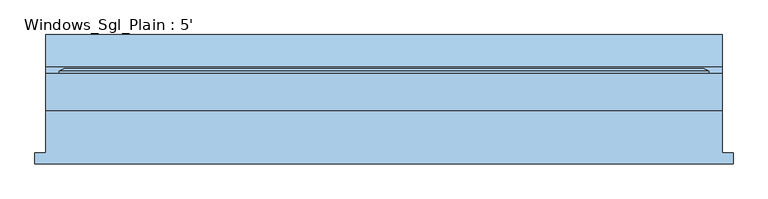
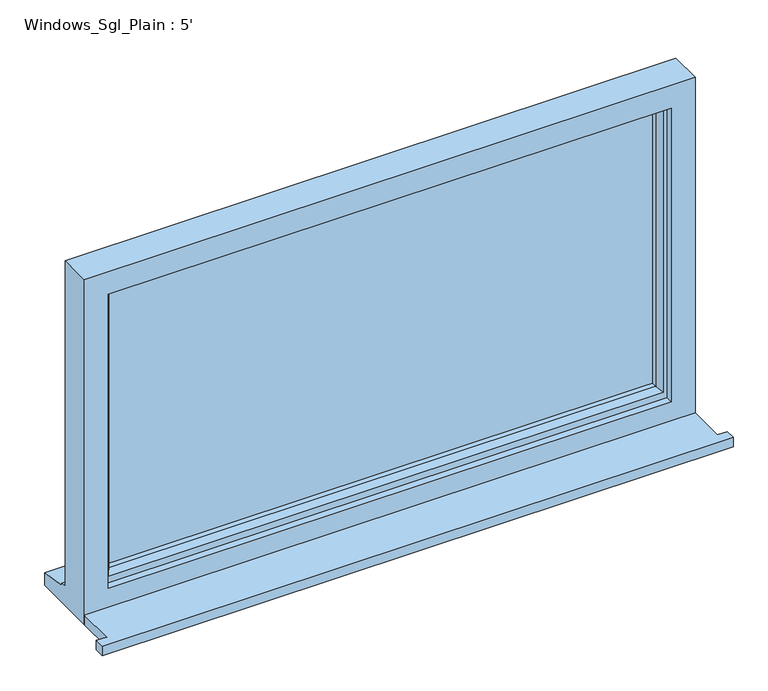
"""IFC4 building model written with IfcOpenShell, lengths in millimetres: window geometry, Windows_Sgl_Plain : 5'."""

from ifc_helpers import new_model, si_unit, frame, origin, place, context, project, spatial, polyline, outline, extrude, faceted_brep, source, transform, mapped, element, save


def windows_sgl_plain_5_79f17ecf(model_context):
    return source(origin(), model_context, "Body", "SolidModel", [
        extrude(outline(polyline([(-787.0, -130.8434322), (-787.0, -105.8434322), (-762.0, -105.8434322), (-762.0, -10.2434322), (762.0, -10.2434322), (762.0, -105.8434322), (787.0, -105.8434322), (787.0, -130.8434322), (-787.0, -130.8434322)])), frame((0.0, 0.0, 1200.0), z_axis=(0.0, 0.0, 1.0), x_axis=(1.0, 0.0, 0.0)), (0.0, 0.0, 1.0), 25.0),
        faceted_brep([(-762.0, -10.2434322, 1200.0), (762.0, -10.2434322, 1200.0), (762.0, -10.2434322, 2110.0), (-762.0, -10.2434322, 2110.0), (-702.0, -10.2434322, 2050.0), (702.0, -10.2434322, 2050.0), (702.0, -10.2434322, 1275.0), (-702.0, -10.2434322, 1275.0), (-762.0, 72.7565678, 2110.0), (-762.0, 72.7565678, 1251.0), (-762.0, 87.7565678, 1249.68767), (-762.0, 87.7565678, 1244.7449676), (-762.0, 160.2565678, 1233.8088847), (-762.0, 160.2565678, 1200.0), (762.0, 72.7565678, 2110.0), (762.0, 72.7565678, 1251.0), (-722.0, 72.7565678, 2070.0), (-722.0, 72.7565678, 1263.0), (722.0, 72.7565678, 1263.0), (722.0, 72.7565678, 2070.0), (-722.0, 7.7565678, 2070.0), (-722.0, 7.7565678, 1263.0), (722.0, 7.7565678, 2070.0), (722.0, 7.7565678, 1263.0), (-702.0, 7.7565678, 2050.0), (-702.0, 7.7565678, 1275.0), (702.0, 7.7565678, 1275.0), (702.0, 7.7565678, 2050.0), (762.0, 160.2565678, 1200.0), (762.0, 160.2565678, 1233.8088847), (762.0, 87.7565678, 1244.7449676), (762.0, 87.7565678, 1249.68767)], [[[0, 1, 2, 3], [4, 5, 6, 7]], [[0, 3, 8, 9, 10, 11, 12, 13]], [[9, 8, 14, 15], [16, 17, 18, 19]], [[17, 16, 20, 21]], [[20, 22, 23, 21], [24, 25, 26, 27]], [[24, 4, 7, 25]], [[3, 2, 14, 8]], [[16, 19, 22, 20]], [[5, 4, 24, 27]], [[15, 14, 2, 1, 28, 29, 30, 31]], [[19, 18, 23, 22]], [[5, 27, 26, 6]], [[28, 1, 0, 13]], [[29, 28, 13, 12]], [[30, 29, 12, 11]], [[31, 30, 11, 10]], [[15, 31, 10, 9]], [[21, 23, 18, 17]], [[7, 6, 26, 25]]]),
        extrude(outline(polyline([(692.0, 36.7565678), (-692.0, 36.7565678), (-692.0, 60.7565678), (692.0, 60.7565678), (692.0, 36.7565678)])), frame((0.0, 0.0, 1293.0), z_axis=(0.0, 0.0, 1.0), x_axis=(1.0, 0.0, 0.0)), (0.0, 0.0, 1.0), 747.0),
        faceted_brep([(-732.0, 72.7565678, 2080.0), (-732.0, 78.5300705, 2080.0), (-732.0, 78.5300705, 1253.0), (-732.0, 72.7565678, 1253.0), (-722.0, 7.7565678, 2070.0), (-722.0, 72.7565678, 2070.0), (-722.0, 72.7565678, 1263.0), (-722.0, 7.7565678, 1263.0), (-682.0, 22.2494677, 2030.0), (-692.1480377, 7.7565678, 2040.1480377), (-692.1480377, 7.7565678, 1292.8519623), (-682.0, 22.2494677, 1303.0), (-682.0, 36.7565678, 2030.0), (-682.0, 36.7565678, 1303.0), (-692.0, 60.7565678, 2040.0), (-692.0, 36.7565678, 2040.0), (-692.0, 36.7565678, 1293.0), (-692.0, 60.7565678, 1293.0), (-682.0, 78.5300705, 2030.0), (-682.0, 60.7565678, 2030.0), (-682.0, 60.7565678, 1303.0), (-682.0, 78.5300705, 1303.0), (-699.4457548, 84.3035732, 2047.4457548), (-699.4457548, 84.3035732, 1285.5542452), (-721.2153903, 84.3035732, 2069.2153903), (-721.2153903, 84.3035732, 1263.7846097), (732.0, 78.5300705, 1253.0), (732.0, 72.7565678, 1253.0), (722.0, 72.7565678, 1263.0), (722.0, 7.7565678, 1263.0), (692.1480377, 7.7565678, 1292.8519623), (682.0, 22.2494677, 1303.0), (682.0, 36.7565678, 1303.0), (692.0, 36.7565678, 1293.0), (692.0, 60.7565678, 1293.0), (682.0, 60.7565678, 1303.0), (682.0, 78.5300705, 1303.0), (699.4457548, 84.3035732, 1285.5542452), (721.2153903, 84.3035732, 1263.7846097), (732.0, 78.5300705, 2080.0), (732.0, 72.7565678, 2080.0), (722.0, 72.7565678, 2070.0), (722.0, 7.7565678, 2070.0), (692.1480377, 7.7565678, 2040.1480377), (682.0, 22.2494677, 2030.0), (682.0, 36.7565678, 2030.0), (692.0, 36.7565678, 2040.0), (692.0, 60.7565678, 2040.0), (682.0, 60.7565678, 2030.0), (682.0, 78.5300705, 2030.0), (699.4457548, 84.3035732, 2047.4457548), (721.2153903, 84.3035732, 2069.2153903)], [[[0, 1, 2, 3]], [[4, 5, 6, 7]], [[8, 9, 10, 11]], [[12, 8, 11, 13]], [[14, 15, 16, 17]], [[18, 19, 20, 21]], [[22, 18, 21, 23]], [[1, 24, 25, 2]], [[3, 2, 26, 27]], [[7, 6, 28, 29]], [[11, 10, 30, 31]], [[13, 11, 31, 32]], [[17, 16, 33, 34]], [[21, 20, 35, 36]], [[23, 21, 36, 37]], [[2, 25, 38, 26]], [[27, 26, 39, 40]], [[29, 28, 41, 42]], [[31, 30, 43, 44]], [[32, 31, 44, 45]], [[34, 33, 46, 47]], [[36, 35, 48, 49]], [[37, 36, 49, 50]], [[26, 38, 51, 39]], [[40, 39, 1, 0]], [[3, 27, 40, 0], [5, 41, 28, 6]], [[42, 41, 5, 4]], [[7, 29, 42, 4], [9, 43, 30, 10]], [[44, 43, 9, 8]], [[45, 44, 8, 12]], [[15, 46, 33, 16], [13, 32, 45, 12]], [[47, 46, 15, 14]], [[17, 34, 47, 14], [19, 48, 35, 20]], [[49, 48, 19, 18]], [[50, 49, 18, 22]], [[24, 51, 38, 25], [23, 37, 50, 22]], [[39, 51, 24, 1]]]),
    ])


if __name__ == "__main__":
    model = new_model("IFC4")
    model_context = context("Model", 3, world=origin())
    ifc_project = project(units=[si_unit("LENGTHUNIT", "METRE", prefix="MILLI")], contexts=[model_context])
    site = spatial("IfcSite", under=ifc_project)
    building = spatial("IfcBuilding", under=site)
    placement = place(None, origin())
    windows_sgl_plain_5_shape = windows_sgl_plain_5_79f17ecf(model_context)
    element("IfcWindow", 1, ObjectType="Windows_Sgl_Plain : 5'", at=placement, inside=building, context=model_context, shape_type="MappedRepresentation", body=[
        mapped(windows_sgl_plain_5_shape, transform((0.0, 0.0, 0.0), x_axis=(1.0, 0.0, 0.0), y_axis=(0.0, 1.0, 0.0), z_axis=(0.0, 0.0, 1.0))),
    ])
    save(model, "model.ifc")

# Revit data of these elements
# Type "Windows_Sgl_Plain : 5'"
#   Type Mark = "67"
#   Operation = "SinglePanel"
#   Construction Type Id = "SGL"
#   Manufacturer = "Revit"
#   Keynote = "L10"
#   Analytic Construction = "Large single-glazed windows"
#   Wrap Layers (Ext) from Ext = 0' - 4.03543"
#   Wrap Layers (Int) from Ext = 0' - 6.98819"
#   Window Board Projection = 0' - 0.98425"
#   Window Board Extension = 0' - 0.98425"
#   Visual Light Transmittance = 0.9
#   Solar Heat Gain Coefficient = 0.86
#   Rough Width = 5' - 0"
#   Rough Height = 2' - 11.82677"
#   Height = 2' - 11.82677"
#   Width = 5' - 0"
#   Heat Transfer Coefficient (U) = 5.5617 W/(m²·K)
#   Glazing Thickness = 0' - 0.94488"
#   FrameOffset - External = 0' - 1.9685"
#   Frame Depth = 0' - 2.55906"
#   Default Head Height = 6' - 11.07087"
#   Cill Depth = 0' - 3.44488"
#   Cavity Closer Width = 0' - 1.9685"
#   Cavity Closer Offset from Ext = 0' - 4.03543"
#   Cavity Closer Depth = 0' - 3.34646"
#   Vis - Cavity Closers = yes
#   Define Thermal Properties by = 1
#   Material Trim = Window Frame
#   Material Glass = Glass
#   Material Frame = Window Frame
#   Wall Closure = (empty or 0)
# Element 1 (IfcWindow, "Windows_Sgl_Plain : 5'")
#   Materials on its faces: "Window Frame", "Glass"
# Materials
#   "Window Frame": colour RGB 249 249 249, transparency 0, Keynote = "L10", Cost = 0
#   "Glass": class "Glass", colour RGB 0 128 192, transparency 0.9, Description = "Soda Lime Glass", Cost = 0
